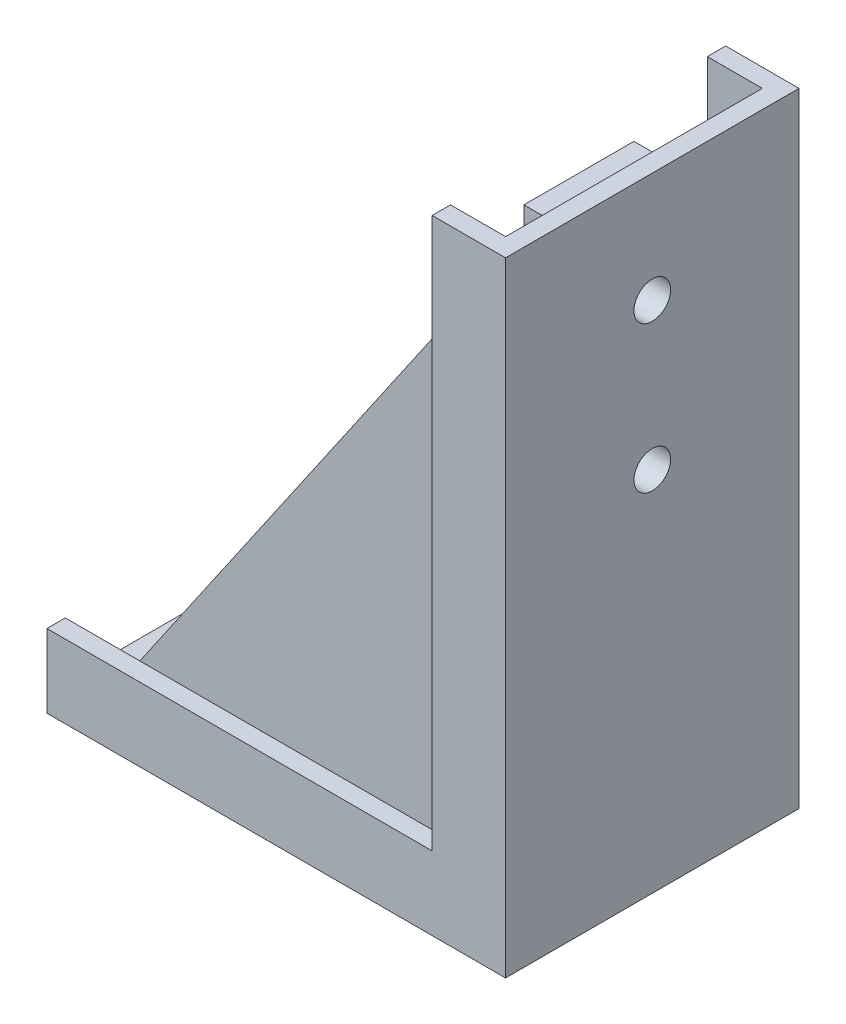
ISO-10303-21;
HEADER;
FILE_DESCRIPTION(('STEP AP214'),'2;1');
FILE_NAME('part.step','',(''),(''),'','','');
FILE_SCHEMA(('AUTOMOTIVE_DESIGN { 1 0 10303 214 1 1 1 1 }'));
ENDSEC;
DATA;
#1=APPLICATION_CONTEXT('core data for automotive mechanical design processes');
#2=APPLICATION_PROTOCOL_DEFINITION('international standard','automotive_design',2000,#1);
#3=PRODUCT_CONTEXT('',#1,'mechanical');
#4=PRODUCT('Part','Part','',(#3));
#5=PRODUCT_RELATED_PRODUCT_CATEGORY('part','',(#4));
#6=PRODUCT_DEFINITION_FORMATION('','',#4);
#7=PRODUCT_DEFINITION_CONTEXT('part definition',#1,'design');
#8=PRODUCT_DEFINITION('design','',#6,#7);
#9=PRODUCT_DEFINITION_SHAPE('','',#8);
#10=(LENGTH_UNIT() NAMED_UNIT(*) SI_UNIT(.MILLI.,.METRE.));
#11=(NAMED_UNIT(*) PLANE_ANGLE_UNIT() SI_UNIT($,.RADIAN.));
#12=(NAMED_UNIT(*) SI_UNIT($,.STERADIAN.) SOLID_ANGLE_UNIT());
#13=UNCERTAINTY_MEASURE_WITH_UNIT(LENGTH_MEASURE(1.E-05),#10,'distance_accuracy_value','');
#14=(GEOMETRIC_REPRESENTATION_CONTEXT(3) GLOBAL_UNCERTAINTY_ASSIGNED_CONTEXT((#13)) GLOBAL_UNIT_ASSIGNED_CONTEXT((#10,
#11,#12)) REPRESENTATION_CONTEXT('',''));
#15=CARTESIAN_POINT('',(0.,0.,0.));
#16=DIRECTION('',(0.,0.,1.));
#17=DIRECTION('',(1.,0.,0.));
#18=AXIS2_PLACEMENT_3D('',#15,#16,#17);
#19=CARTESIAN_POINT('',(-1.25,1.25,20.));
#20=DIRECTION('',(1.,0.,0.));
#21=DIRECTION('',(0.,1.,0.));
#22=AXIS2_PLACEMENT_3D('',#19,#20,#21);
#23=PLANE('',#22);
#24=DIRECTION('',(0.,-1.,0.));
#25=VECTOR('',#24,1.);
#26=CARTESIAN_POINT('',(-1.25,40.,6.25));
#27=LINE('',#26,#25);
#28=CARTESIAN_POINT('',(-1.25,40.,6.25));
#29=VERTEX_POINT('',#28);
#30=CARTESIAN_POINT('',(-1.25,17.5,6.25));
#31=VERTEX_POINT('',#30);
#32=EDGE_CURVE('E212',#29,#31,#27,.T.);
#33=ORIENTED_EDGE('',*,*,#32,.F.);
#34=DIRECTION('',(0.,0.,-1.));
#35=VECTOR('',#34,1.);
#36=CARTESIAN_POINT('',(-1.25,40.,6.25));
#37=LINE('',#36,#35);
#38=CARTESIAN_POINT('',(-1.25,40.,13.75));
#39=VERTEX_POINT('',#38);
#40=EDGE_CURVE('E206',#39,#29,#37,.T.);
#41=ORIENTED_EDGE('',*,*,#40,.F.);
#42=DIRECTION('',(0.,1.,0.));
#43=VECTOR('',#42,1.);
#44=CARTESIAN_POINT('',(-1.25,40.,13.75));
#45=LINE('',#44,#43);
#46=CARTESIAN_POINT('',(-1.25,17.5,13.75));
#47=VERTEX_POINT('',#46);
#48=EDGE_CURVE('E62',#47,#39,#45,.T.);
#49=ORIENTED_EDGE('',*,*,#48,.F.);
#50=DIRECTION('',(0.,0.,1.));
#51=VECTOR('',#50,1.);
#52=CARTESIAN_POINT('',(-1.25,17.5,6.25));
#53=LINE('',#52,#51);
#54=EDGE_CURVE('E57',#31,#47,#53,.T.);
#55=ORIENTED_EDGE('',*,*,#54,.F.);
#56=EDGE_LOOP('',(#33,#41,#49,#55));
#57=FACE_BOUND('',#56,.T.);
#58=DIRECTION('',(0.,0.,1.));
#59=VECTOR('',#58,1.);
#60=CARTESIAN_POINT('',(-1.25,41.25,17.5));
#61=LINE('',#60,#59);
#62=CARTESIAN_POINT('',(-1.25,41.25,17.5));
#63=VERTEX_POINT('',#62);
#64=CARTESIAN_POINT('',(-1.25,41.25,18.75));
#65=VERTEX_POINT('',#64);
#66=EDGE_CURVE('E228',#63,#65,#61,.T.);
#67=ORIENTED_EDGE('',*,*,#66,.T.);
#68=DIRECTION('',(0.,-1.,0.));
#69=VECTOR('',#68,1.);
#70=CARTESIAN_POINT('',(-1.25,42.5,18.75));
#71=LINE('',#70,#69);
#72=CARTESIAN_POINT('',(-1.25,42.5,18.75));
#73=VERTEX_POINT('',#72);
#74=EDGE_CURVE('E283',#73,#65,#71,.T.);
#75=ORIENTED_EDGE('',*,*,#74,.F.);
#76=DIRECTION('',(0.,0.,-1.));
#77=VECTOR('',#76,1.);
#78=CARTESIAN_POINT('',(-1.25,42.5,20.));
#79=LINE('',#78,#77);
#80=CARTESIAN_POINT('',(-1.25,42.5,1.25));
#81=VERTEX_POINT('',#80);
#82=EDGE_CURVE('E48',#73,#81,#79,.T.);
#83=ORIENTED_EDGE('',*,*,#82,.T.);
#84=DIRECTION('',(0.,-1.,0.));
#85=VECTOR('',#84,1.);
#86=CARTESIAN_POINT('',(-1.25,1.25,1.25));
#87=LINE('',#86,#85);
#88=CARTESIAN_POINT('',(-1.25,41.25,1.25));
#89=VERTEX_POINT('',#88);
#90=EDGE_CURVE('E278',#81,#89,#87,.T.);
#91=ORIENTED_EDGE('',*,*,#90,.T.);
#92=DIRECTION('',(0.,0.,-1.));
#93=VECTOR('',#92,1.);
#94=CARTESIAN_POINT('',(-1.25,41.25,2.5));
#95=LINE('',#94,#93);
#96=CARTESIAN_POINT('',(-1.25,41.25,2.5));
#97=VERTEX_POINT('',#96);
#98=EDGE_CURVE('E250',#97,#89,#95,.T.);
#99=ORIENTED_EDGE('',*,*,#98,.F.);
#100=DIRECTION('',(0.,-1.,0.));
#101=VECTOR('',#100,1.);
#102=CARTESIAN_POINT('',(-1.25,41.25,2.5));
#103=LINE('',#102,#101);
#104=CARTESIAN_POINT('',(-1.25,1.25,2.5));
#105=VERTEX_POINT('',#104);
#106=EDGE_CURVE('E239',#97,#105,#103,.T.);
#107=ORIENTED_EDGE('',*,*,#106,.T.);
#108=DIRECTION('',(0.,0.,-1.));
#109=VECTOR('',#108,1.);
#110=CARTESIAN_POINT('',(-1.25,1.25,20.));
#111=LINE('',#110,#109);
#112=CARTESIAN_POINT('',(-1.25,1.25,17.5));
#113=VERTEX_POINT('',#112);
#114=EDGE_CURVE('E341',#113,#105,#111,.T.);
#115=ORIENTED_EDGE('',*,*,#114,.F.);
#116=DIRECTION('',(0.,-1.,0.));
#117=VECTOR('',#116,1.);
#118=CARTESIAN_POINT('',(-1.25,1.25,17.5));
#119=LINE('',#118,#117);
#120=EDGE_CURVE('E221',#63,#113,#119,.T.);
#121=ORIENTED_EDGE('',*,*,#120,.F.);
#122=EDGE_LOOP('',(#67,#75,#83,#91,#99,#107,#115,#121));
#123=FACE_BOUND('',#122,.T.);
#124=ADVANCED_FACE('F39',(#57,#123),#23,.F.);
#125=CARTESIAN_POINT('',(-31.25,1.25,20.));
#126=DIRECTION('',(0.,-1.,0.));
#127=DIRECTION('',(1.,0.,0.));
#128=AXIS2_PLACEMENT_3D('',#125,#126,#127);
#129=PLANE('',#128);
#130=DIRECTION('',(0.,0.,1.));
#131=VECTOR('',#130,1.);
#132=CARTESIAN_POINT('',(-28.75,1.25,17.5));
#133=LINE('',#132,#131);
#134=CARTESIAN_POINT('',(-28.75,1.25,17.5));
#135=VERTEX_POINT('',#134);
#136=CARTESIAN_POINT('',(-28.75,1.25,18.75));
#137=VERTEX_POINT('',#136);
#138=EDGE_CURVE('E233',#135,#137,#133,.T.);
#139=ORIENTED_EDGE('',*,*,#138,.F.);
#140=DIRECTION('',(-1.,0.,0.));
#141=VECTOR('',#140,1.);
#142=CARTESIAN_POINT('',(-28.75,1.25,17.5));
#143=LINE('',#142,#141);
#144=EDGE_CURVE('E224',#113,#135,#143,.T.);
#145=ORIENTED_EDGE('',*,*,#144,.F.);
#146=ORIENTED_EDGE('',*,*,#114,.T.);
#147=DIRECTION('',(-1.,0.,0.));
#148=VECTOR('',#147,1.);
#149=CARTESIAN_POINT('',(-1.25,1.25,2.5));
#150=LINE('',#149,#148);
#151=CARTESIAN_POINT('',(-28.75,1.24999999999999,2.5));
#152=VERTEX_POINT('',#151);
#153=EDGE_CURVE('E234',#105,#152,#150,.T.);
#154=ORIENTED_EDGE('',*,*,#153,.T.);
#155=DIRECTION('',(0.,0.,-1.));
#156=VECTOR('',#155,1.);
#157=CARTESIAN_POINT('',(-28.75,1.24999999999999,2.5));
#158=LINE('',#157,#156);
#159=CARTESIAN_POINT('',(-28.75,1.24999999999999,1.25));
#160=VERTEX_POINT('',#159);
#161=EDGE_CURVE('E243',#152,#160,#158,.T.);
#162=ORIENTED_EDGE('',*,*,#161,.T.);
#163=DIRECTION('',(-1.,0.,0.));
#164=VECTOR('',#163,1.);
#165=CARTESIAN_POINT('',(-31.25,1.25,1.25));
#166=LINE('',#165,#164);
#167=CARTESIAN_POINT('',(-31.25,1.25,1.25));
#168=VERTEX_POINT('',#167);
#169=EDGE_CURVE('E274',#160,#168,#166,.T.);
#170=ORIENTED_EDGE('',*,*,#169,.T.);
#171=DIRECTION('',(0.,0.,-1.));
#172=VECTOR('',#171,1.);
#173=CARTESIAN_POINT('',(-31.25,1.25,20.));
#174=LINE('',#173,#172);
#175=CARTESIAN_POINT('',(-31.25,1.25,18.75));
#176=VERTEX_POINT('',#175);
#177=EDGE_CURVE('E342',#176,#168,#174,.T.);
#178=ORIENTED_EDGE('',*,*,#177,.F.);
#179=DIRECTION('',(-1.,0.,0.));
#180=VECTOR('',#179,1.);
#181=CARTESIAN_POINT('',(-1.25,1.25,18.75));
#182=LINE('',#181,#180);
#183=EDGE_CURVE('E287',#137,#176,#182,.T.);
#184=ORIENTED_EDGE('',*,*,#183,.F.);
#185=EDGE_LOOP('',(#139,#145,#146,#154,#162,#170,#178,#184));
#186=FACE_BOUND('',#185,.T.);
#187=ADVANCED_FACE('F387',(#186),#129,.F.);
#188=CARTESIAN_POINT('',(0.,0.,18.75));
#189=DIRECTION('',(0.,0.,-1.));
#190=DIRECTION('',(-1.,0.,0.));
#191=AXIS2_PLACEMENT_3D('',#188,#189,#190);
#192=PLANE('',#191);
#193=ORIENTED_EDGE('',*,*,#74,.T.);
#194=DIRECTION('',(-0.566528822887065,-0.824041924199368,0.));
#195=VECTOR('',#194,1.);
#196=CARTESIAN_POINT('',(-20.106100795756,13.8229442970822,18.75));
#197=LINE('',#196,#195);
#198=CARTESIAN_POINT('',(-5.,35.7954545454545,18.75));
#199=VERTEX_POINT('',#198);
#200=EDGE_CURVE('E11',#65,#199,#197,.T.);
#201=ORIENTED_EDGE('',*,*,#200,.T.);
#202=DIRECTION('',(0.,-1.,0.));
#203=VECTOR('',#202,1.);
#204=CARTESIAN_POINT('',(-5.,42.5,18.75));
#205=LINE('',#204,#203);
#206=CARTESIAN_POINT('',(-5.,42.5,18.75));
#207=VERTEX_POINT('',#206);
#208=EDGE_CURVE('E296',#207,#199,#205,.T.);
#209=ORIENTED_EDGE('',*,*,#208,.F.);
#210=DIRECTION('',(-1.,0.,0.));
#211=VECTOR('',#210,1.);
#212=CARTESIAN_POINT('',(-1.25,42.5,18.75));
#213=LINE('',#212,#211);
#214=EDGE_CURVE('E301',#73,#207,#213,.T.);
#215=ORIENTED_EDGE('',*,*,#214,.F.);
#216=EDGE_LOOP('',(#193,#201,#209,#215));
#217=FACE_BOUND('',#216,.T.);
#218=ADVANCED_FACE('F395',(#217),#192,.T.);
#219=DIRECTION('',(-1.,0.,0.));
#220=VECTOR('',#219,1.);
#221=CARTESIAN_POINT('',(-5.,5.,18.75));
#222=LINE('',#221,#220);
#223=CARTESIAN_POINT('',(-26.171875,5.,18.75));
#224=VERTEX_POINT('',#223);
#225=CARTESIAN_POINT('',(-31.25,5.,18.75));
#226=VERTEX_POINT('',#225);
#227=EDGE_CURVE('E291',#224,#226,#222,.T.);
#228=ORIENTED_EDGE('',*,*,#227,.F.);
#229=DIRECTION('',(0.566528822887065,0.824041924199368,0.));
#230=VECTOR('',#229,1.);
#231=CARTESIAN_POINT('',(-1.25,41.25,18.75));
#232=LINE('',#231,#230);
#233=EDGE_CURVE('E213',#137,#224,#232,.T.);
#234=ORIENTED_EDGE('',*,*,#233,.F.);
#235=ORIENTED_EDGE('',*,*,#183,.T.);
#236=DIRECTION('',(0.,-1.,0.));
#237=VECTOR('',#236,1.);
#238=CARTESIAN_POINT('',(-31.25,5.,18.75));
#239=LINE('',#238,#237);
#240=EDGE_CURVE('E290',#226,#176,#239,.T.);
#241=ORIENTED_EDGE('',*,*,#240,.F.);
#242=EDGE_LOOP('',(#228,#234,#235,#241));
#243=FACE_BOUND('',#242,.T.);
#244=ADVANCED_FACE('F430',(#243),#192,.T.);
#245=CARTESIAN_POINT('',(0.,0.,1.25));
#246=DIRECTION('',(0.,0.,1.));
#247=DIRECTION('',(1.,0.,0.));
#248=AXIS2_PLACEMENT_3D('',#245,#246,#247);
#249=PLANE('',#248);
#250=DIRECTION('',(0.566528822887065,0.824041924199368,0.));
#251=VECTOR('',#250,1.);
#252=CARTESIAN_POINT('',(-28.75,1.24999999999999,1.25));
#253=LINE('',#252,#251);
#254=CARTESIAN_POINT('',(-5.,35.7954545454545,1.25));
#255=VERTEX_POINT('',#254);
#256=EDGE_CURVE('E231',#255,#89,#253,.T.);
#257=ORIENTED_EDGE('',*,*,#256,.T.);
#258=ORIENTED_EDGE('',*,*,#90,.F.);
#259=DIRECTION('',(1.,0.,0.));
#260=VECTOR('',#259,1.);
#261=CARTESIAN_POINT('',(-1.25,42.5,1.25));
#262=LINE('',#261,#260);
#263=CARTESIAN_POINT('',(-5.,42.5,1.25));
#264=VERTEX_POINT('',#263);
#265=EDGE_CURVE('E262',#264,#81,#262,.T.);
#266=ORIENTED_EDGE('',*,*,#265,.F.);
#267=DIRECTION('',(0.,1.,0.));
#268=VECTOR('',#267,1.);
#269=CARTESIAN_POINT('',(-5.,42.5,1.25));
#270=LINE('',#269,#268);
#271=EDGE_CURVE('E256',#255,#264,#270,.T.);
#272=ORIENTED_EDGE('',*,*,#271,.F.);
#273=EDGE_LOOP('',(#257,#258,#266,#272));
#274=FACE_BOUND('',#273,.T.);
#275=ADVANCED_FACE('F441',(#274),#249,.T.);
#276=CARTESIAN_POINT('',(-1.25,42.5,20.));
#277=DIRECTION('',(0.,-1.,0.));
#278=DIRECTION('',(0.,0.,-1.));
#279=AXIS2_PLACEMENT_3D('',#276,#277,#278);
#280=PLANE('',#279);
#281=DIRECTION('',(0.,0.,-1.));
#282=VECTOR('',#281,1.);
#283=CARTESIAN_POINT('',(0.,42.5,20.));
#284=LINE('',#283,#282);
#285=CARTESIAN_POINT('',(0.,42.5,20.));
#286=VERTEX_POINT('',#285);
#287=CARTESIAN_POINT('',(0.,42.5,0.));
#288=VERTEX_POINT('',#287);
#289=EDGE_CURVE('E326',#286,#288,#284,.T.);
#290=ORIENTED_EDGE('',*,*,#289,.T.);
#291=DIRECTION('',(-1.,0.,0.));
#292=VECTOR('',#291,1.);
#293=CARTESIAN_POINT('',(-1.25,42.5,0.));
#294=LINE('',#293,#292);
#295=CARTESIAN_POINT('',(-5.,42.5,0.));
#296=VERTEX_POINT('',#295);
#297=EDGE_CURVE('E317',#288,#296,#294,.T.);
#298=ORIENTED_EDGE('',*,*,#297,.T.);
#299=DIRECTION('',(0.,0.,-1.));
#300=VECTOR('',#299,1.);
#301=CARTESIAN_POINT('',(-5.,42.5,1.25));
#302=LINE('',#301,#300);
#303=EDGE_CURVE('E272',#264,#296,#302,.T.);
#304=ORIENTED_EDGE('',*,*,#303,.F.);
#305=ORIENTED_EDGE('',*,*,#265,.T.);
#306=ORIENTED_EDGE('',*,*,#82,.F.);
#307=ORIENTED_EDGE('',*,*,#214,.T.);
#308=DIRECTION('',(0.,0.,1.));
#309=VECTOR('',#308,1.);
#310=CARTESIAN_POINT('',(-5.,42.5,18.75));
#311=LINE('',#310,#309);
#312=CARTESIAN_POINT('',(-5.,42.5,20.));
#313=VERTEX_POINT('',#312);
#314=EDGE_CURVE('E302',#207,#313,#311,.T.);
#315=ORIENTED_EDGE('',*,*,#314,.T.);
#316=DIRECTION('',(-1.,0.,0.));
#317=VECTOR('',#316,1.);
#318=CARTESIAN_POINT('',(-1.25,42.5,20.));
#319=LINE('',#318,#317);
#320=EDGE_CURVE('E320',#286,#313,#319,.T.);
#321=ORIENTED_EDGE('',*,*,#320,.F.);
#322=EDGE_LOOP('',(#290,#298,#304,#305,#306,#307,#315,#321));
#323=FACE_BOUND('',#322,.T.);
#324=ADVANCED_FACE('F41',(#323),#280,.F.);
#325=CARTESIAN_POINT('',(-31.25,0.,20.));
#326=DIRECTION('',(1.,0.,0.));
#327=DIRECTION('',(0.,0.,-1.));
#328=AXIS2_PLACEMENT_3D('',#325,#326,#327);
#329=PLANE('',#328);
#330=ORIENTED_EDGE('',*,*,#177,.T.);
#331=DIRECTION('',(0.,1.,0.));
#332=VECTOR('',#331,1.);
#333=CARTESIAN_POINT('',(-31.25,1.25,1.25));
#334=LINE('',#333,#332);
#335=CARTESIAN_POINT('',(-31.25,5.,1.25));
#336=VERTEX_POINT('',#335);
#337=EDGE_CURVE('E255',#168,#336,#334,.T.);
#338=ORIENTED_EDGE('',*,*,#337,.T.);
#339=DIRECTION('',(0.,0.,-1.));
#340=VECTOR('',#339,1.);
#341=CARTESIAN_POINT('',(-31.25,5.,1.25));
#342=LINE('',#341,#340);
#343=CARTESIAN_POINT('',(-31.25,5.,0.));
#344=VERTEX_POINT('',#343);
#345=EDGE_CURVE('E266',#336,#344,#342,.T.);
#346=ORIENTED_EDGE('',*,*,#345,.T.);
#347=DIRECTION('',(0.,-1.,0.));
#348=VECTOR('',#347,1.);
#349=CARTESIAN_POINT('',(-31.25,0.,0.));
#350=LINE('',#349,#348);
#351=CARTESIAN_POINT('',(-31.25,0.,0.));
#352=VERTEX_POINT('',#351);
#353=EDGE_CURVE('E327',#344,#352,#350,.T.);
#354=ORIENTED_EDGE('',*,*,#353,.T.);
#355=DIRECTION('',(0.,0.,-1.));
#356=VECTOR('',#355,1.);
#357=CARTESIAN_POINT('',(-31.25,0.,20.));
#358=LINE('',#357,#356);
#359=CARTESIAN_POINT('',(-31.25,0.,20.));
#360=VERTEX_POINT('',#359);
#361=EDGE_CURVE('E339',#360,#352,#358,.T.);
#362=ORIENTED_EDGE('',*,*,#361,.F.);
#363=DIRECTION('',(0.,-1.,0.));
#364=VECTOR('',#363,1.);
#365=CARTESIAN_POINT('',(-31.25,0.,20.));
#366=LINE('',#365,#364);
#367=CARTESIAN_POINT('',(-31.25,5.,20.));
#368=VERTEX_POINT('',#367);
#369=EDGE_CURVE('E316',#368,#360,#366,.T.);
#370=ORIENTED_EDGE('',*,*,#369,.F.);
#371=DIRECTION('',(0.,0.,1.));
#372=VECTOR('',#371,1.);
#373=CARTESIAN_POINT('',(-31.25,5.,18.75));
#374=LINE('',#373,#372);
#375=EDGE_CURVE('E312',#226,#368,#374,.T.);
#376=ORIENTED_EDGE('',*,*,#375,.F.);
#377=ORIENTED_EDGE('',*,*,#240,.T.);
#378=EDGE_LOOP('',(#330,#338,#346,#354,#362,#370,#376,#377));
#379=FACE_BOUND('',#378,.T.);
#380=ADVANCED_FACE('F397',(#379),#329,.F.);
#381=CARTESIAN_POINT('',(0.,0.,20.));
#382=DIRECTION('',(0.,1.,0.));
#383=DIRECTION('',(0.,0.,1.));
#384=AXIS2_PLACEMENT_3D('',#381,#382,#383);
#385=PLANE('',#384);
#386=ORIENTED_EDGE('',*,*,#361,.T.);
#387=DIRECTION('',(1.,0.,0.));
#388=VECTOR('',#387,1.);
#389=CARTESIAN_POINT('',(0.,0.,0.));
#390=LINE('',#389,#388);
#391=CARTESIAN_POINT('',(0.,0.,0.));
#392=VERTEX_POINT('',#391);
#393=EDGE_CURVE('E331',#352,#392,#390,.T.);
#394=ORIENTED_EDGE('',*,*,#393,.T.);
#395=DIRECTION('',(0.,0.,-1.));
#396=VECTOR('',#395,1.);
#397=CARTESIAN_POINT('',(0.,0.,20.));
#398=LINE('',#397,#396);
#399=CARTESIAN_POINT('',(0.,0.,20.));
#400=VERTEX_POINT('',#399);
#401=EDGE_CURVE('E340',#400,#392,#398,.T.);
#402=ORIENTED_EDGE('',*,*,#401,.F.);
#403=DIRECTION('',(1.,0.,0.));
#404=VECTOR('',#403,1.);
#405=CARTESIAN_POINT('',(0.,0.,20.));
#406=LINE('',#405,#404);
#407=EDGE_CURVE('E325',#360,#400,#406,.T.);
#408=ORIENTED_EDGE('',*,*,#407,.F.);
#409=EDGE_LOOP('',(#386,#394,#402,#408));
#410=FACE_BOUND('',#409,.T.);
#411=ADVANCED_FACE('F400',(#410),#385,.F.);
#412=CARTESIAN_POINT('',(0.,42.5,20.));
#413=DIRECTION('',(-1.,0.,0.));
#414=DIRECTION('',(0.,-1.,0.));
#415=AXIS2_PLACEMENT_3D('',#412,#413,#414);
#416=PLANE('',#415);
#417=CARTESIAN_POINT('',(0.,35.,10.));
#418=DIRECTION('',(-1.,0.,0.));
#419=DIRECTION('',(0.,-1.,0.));
#420=AXIS2_PLACEMENT_3D('',#417,#418,#419);
#421=CIRCLE('',#420,1.25);
#422=CARTESIAN_POINT('',(0.,33.75,10.));
#423=VERTEX_POINT('',#422);
#424=EDGE_CURVE('E43',#423,#423,#421,.T.);
#425=ORIENTED_EDGE('',*,*,#424,.T.);
#426=EDGE_LOOP('',(#425));
#427=FACE_BOUND('',#426,.T.);
#428=CARTESIAN_POINT('',(0.,25.,10.));
#429=DIRECTION('',(-1.,0.,0.));
#430=DIRECTION('',(0.,-1.,0.));
#431=AXIS2_PLACEMENT_3D('',#428,#429,#430);
#432=CIRCLE('',#431,1.25);
#433=CARTESIAN_POINT('',(0.,23.75,10.));
#434=VERTEX_POINT('',#433);
#435=EDGE_CURVE('E346',#434,#434,#432,.T.);
#436=ORIENTED_EDGE('',*,*,#435,.T.);
#437=EDGE_LOOP('',(#436));
#438=FACE_BOUND('',#437,.T.);
#439=ORIENTED_EDGE('',*,*,#401,.T.);
#440=DIRECTION('',(0.,1.,0.));
#441=VECTOR('',#440,1.);
#442=CARTESIAN_POINT('',(0.,42.5,0.));
#443=LINE('',#442,#441);
#444=EDGE_CURVE('E318',#392,#288,#443,.T.);
#445=ORIENTED_EDGE('',*,*,#444,.T.);
#446=ORIENTED_EDGE('',*,*,#289,.F.);
#447=DIRECTION('',(0.,1.,0.));
#448=VECTOR('',#447,1.);
#449=CARTESIAN_POINT('',(0.,42.5,20.));
#450=LINE('',#449,#448);
#451=EDGE_CURVE('E321',#400,#286,#450,.T.);
#452=ORIENTED_EDGE('',*,*,#451,.F.);
#453=EDGE_LOOP('',(#439,#445,#446,#452));
#454=FACE_BOUND('',#453,.T.);
#455=ADVANCED_FACE('F404',(#427,#438,#454),#416,.F.);
#456=CARTESIAN_POINT('',(0.,0.,20.));
#457=DIRECTION('',(0.,0.,-1.));
#458=DIRECTION('',(-1.,0.,0.));
#459=AXIS2_PLACEMENT_3D('',#456,#457,#458);
#460=PLANE('',#459);
#461=ORIENTED_EDGE('',*,*,#320,.T.);
#462=DIRECTION('',(0.,-1.,0.));
#463=VECTOR('',#462,1.);
#464=CARTESIAN_POINT('',(-5.,42.5,20.));
#465=LINE('',#464,#463);
#466=CARTESIAN_POINT('',(-5.,5.,20.));
#467=VERTEX_POINT('',#466);
#468=EDGE_CURVE('E289',#313,#467,#465,.T.);
#469=ORIENTED_EDGE('',*,*,#468,.T.);
#470=DIRECTION('',(-1.,0.,0.));
#471=VECTOR('',#470,1.);
#472=CARTESIAN_POINT('',(-5.,5.,20.));
#473=LINE('',#472,#471);
#474=EDGE_CURVE('E282',#467,#368,#473,.T.);
#475=ORIENTED_EDGE('',*,*,#474,.T.);
#476=ORIENTED_EDGE('',*,*,#369,.T.);
#477=ORIENTED_EDGE('',*,*,#407,.T.);
#478=ORIENTED_EDGE('',*,*,#451,.T.);
#479=EDGE_LOOP('',(#461,#469,#475,#476,#477,#478));
#480=FACE_BOUND('',#479,.T.);
#481=ADVANCED_FACE('F409',(#480),#460,.F.);
#482=CARTESIAN_POINT('',(0.,0.,0.));
#483=DIRECTION('',(0.,0.,-1.));
#484=DIRECTION('',(-1.,0.,0.));
#485=AXIS2_PLACEMENT_3D('',#482,#483,#484);
#486=PLANE('',#485);
#487=ORIENTED_EDGE('',*,*,#297,.F.);
#488=ORIENTED_EDGE('',*,*,#444,.F.);
#489=ORIENTED_EDGE('',*,*,#393,.F.);
#490=ORIENTED_EDGE('',*,*,#353,.F.);
#491=DIRECTION('',(1.,0.,0.));
#492=VECTOR('',#491,1.);
#493=CARTESIAN_POINT('',(-5.,5.,0.));
#494=LINE('',#493,#492);
#495=CARTESIAN_POINT('',(-5.,5.,0.));
#496=VERTEX_POINT('',#495);
#497=EDGE_CURVE('E248',#344,#496,#494,.T.);
#498=ORIENTED_EDGE('',*,*,#497,.T.);
#499=DIRECTION('',(0.,1.,0.));
#500=VECTOR('',#499,1.);
#501=CARTESIAN_POINT('',(-5.,42.5,0.));
#502=LINE('',#501,#500);
#503=EDGE_CURVE('E253',#496,#296,#502,.T.);
#504=ORIENTED_EDGE('',*,*,#503,.T.);
#505=EDGE_LOOP('',(#487,#488,#489,#490,#498,#504));
#506=FACE_BOUND('',#505,.T.);
#507=ADVANCED_FACE('F406',(#506),#486,.T.);
#508=CARTESIAN_POINT('',(-5.,5.,18.75));
#509=DIRECTION('',(0.,1.,0.));
#510=DIRECTION('',(-1.,0.,0.));
#511=AXIS2_PLACEMENT_3D('',#508,#509,#510);
#512=PLANE('',#511);
#513=ORIENTED_EDGE('',*,*,#474,.F.);
#514=DIRECTION('',(0.,0.,1.));
#515=VECTOR('',#514,1.);
#516=CARTESIAN_POINT('',(-5.,5.,18.75));
#517=LINE('',#516,#515);
#518=CARTESIAN_POINT('',(-5.,5.,18.75));
#519=VERTEX_POINT('',#518);
#520=EDGE_CURVE('E311',#519,#467,#517,.T.);
#521=ORIENTED_EDGE('',*,*,#520,.F.);
#522=EDGE_CURVE('E295',#519,#224,#222,.T.);
#523=ORIENTED_EDGE('',*,*,#522,.T.);
#524=ORIENTED_EDGE('',*,*,#227,.T.);
#525=ORIENTED_EDGE('',*,*,#375,.T.);
#526=EDGE_LOOP('',(#513,#521,#523,#524,#525));
#527=FACE_BOUND('',#526,.T.);
#528=ADVANCED_FACE('F415',(#527),#512,.T.);
#529=CARTESIAN_POINT('',(-5.,42.5,18.75));
#530=DIRECTION('',(-1.,0.,0.));
#531=DIRECTION('',(0.,-1.,0.));
#532=AXIS2_PLACEMENT_3D('',#529,#530,#531);
#533=PLANE('',#532);
#534=ORIENTED_EDGE('',*,*,#468,.F.);
#535=ORIENTED_EDGE('',*,*,#314,.F.);
#536=ORIENTED_EDGE('',*,*,#208,.T.);
#537=EDGE_CURVE('E300',#199,#519,#205,.T.);
#538=ORIENTED_EDGE('',*,*,#537,.T.);
#539=ORIENTED_EDGE('',*,*,#520,.T.);
#540=EDGE_LOOP('',(#534,#535,#536,#538,#539));
#541=FACE_BOUND('',#540,.T.);
#542=ADVANCED_FACE('F418',(#541),#533,.T.);
#543=CARTESIAN_POINT('',(-26.171875,5.,1.25));
#544=VERTEX_POINT('',#543);
#545=EDGE_CURVE('E238',#160,#544,#253,.T.);
#546=ORIENTED_EDGE('',*,*,#545,.T.);
#547=DIRECTION('',(1.,0.,0.));
#548=VECTOR('',#547,1.);
#549=CARTESIAN_POINT('',(-5.,5.,1.25));
#550=LINE('',#549,#548);
#551=EDGE_CURVE('E257',#336,#544,#550,.T.);
#552=ORIENTED_EDGE('',*,*,#551,.F.);
#553=ORIENTED_EDGE('',*,*,#337,.F.);
#554=ORIENTED_EDGE('',*,*,#169,.F.);
#555=EDGE_LOOP('',(#546,#552,#553,#554));
#556=FACE_BOUND('',#555,.T.);
#557=ADVANCED_FACE('F421',(#556),#249,.T.);
#558=CARTESIAN_POINT('',(-5.,42.5,1.25));
#559=DIRECTION('',(-1.,0.,0.));
#560=DIRECTION('',(0.,-1.,0.));
#561=AXIS2_PLACEMENT_3D('',#558,#559,#560);
#562=PLANE('',#561);
#563=ORIENTED_EDGE('',*,*,#503,.F.);
#564=DIRECTION('',(0.,0.,-1.));
#565=VECTOR('',#564,1.);
#566=CARTESIAN_POINT('',(-5.,5.,1.25));
#567=LINE('',#566,#565);
#568=CARTESIAN_POINT('',(-5.,5.,1.25));
#569=VERTEX_POINT('',#568);
#570=EDGE_CURVE('E273',#569,#496,#567,.T.);
#571=ORIENTED_EDGE('',*,*,#570,.F.);
#572=EDGE_CURVE('E258',#569,#255,#270,.T.);
#573=ORIENTED_EDGE('',*,*,#572,.T.);
#574=ORIENTED_EDGE('',*,*,#271,.T.);
#575=ORIENTED_EDGE('',*,*,#303,.T.);
#576=EDGE_LOOP('',(#563,#571,#573,#574,#575));
#577=FACE_BOUND('',#576,.T.);
#578=ADVANCED_FACE('F433',(#577),#562,.T.);
#579=CARTESIAN_POINT('',(-5.,5.,1.25));
#580=DIRECTION('',(0.,1.,0.));
#581=DIRECTION('',(-1.,0.,0.));
#582=AXIS2_PLACEMENT_3D('',#579,#580,#581);
#583=PLANE('',#582);
#584=ORIENTED_EDGE('',*,*,#497,.F.);
#585=ORIENTED_EDGE('',*,*,#345,.F.);
#586=ORIENTED_EDGE('',*,*,#551,.T.);
#587=EDGE_CURVE('E251',#544,#569,#550,.T.);
#588=ORIENTED_EDGE('',*,*,#587,.T.);
#589=ORIENTED_EDGE('',*,*,#570,.T.);
#590=EDGE_LOOP('',(#584,#585,#586,#588,#589));
#591=FACE_BOUND('',#590,.T.);
#592=ADVANCED_FACE('F429',(#591),#583,.T.);
#593=CARTESIAN_POINT('',(-28.75,1.24999999999999,2.5));
#594=DIRECTION('',(-0.824041924199368,0.566528822887065,0.));
#595=DIRECTION('',(-0.566528822887065,-0.824041924199368,0.));
#596=AXIS2_PLACEMENT_3D('',#593,#594,#595);
#597=PLANE('',#596);
#598=ORIENTED_EDGE('',*,*,#545,.F.);
#599=ORIENTED_EDGE('',*,*,#161,.F.);
#600=DIRECTION('',(0.566528822887065,0.824041924199368,0.));
#601=VECTOR('',#600,1.);
#602=CARTESIAN_POINT('',(-28.75,1.24999999999999,2.5));
#603=LINE('',#602,#601);
#604=EDGE_CURVE('E240',#152,#97,#603,.T.);
#605=ORIENTED_EDGE('',*,*,#604,.T.);
#606=ORIENTED_EDGE('',*,*,#98,.T.);
#607=ORIENTED_EDGE('',*,*,#256,.F.);
#608=EDGE_CURVE('E246',#544,#255,#253,.T.);
#609=ORIENTED_EDGE('',*,*,#608,.F.);
#610=EDGE_LOOP('',(#598,#599,#605,#606,#607,#609));
#611=FACE_BOUND('',#610,.T.);
#612=ADVANCED_FACE('F435',(#611),#597,.T.);
#613=CARTESIAN_POINT('',(0.,0.,2.5));
#614=DIRECTION('',(0.,0.,1.));
#615=DIRECTION('',(1.,0.,0.));
#616=AXIS2_PLACEMENT_3D('',#613,#614,#615);
#617=PLANE('',#616);
#618=ORIENTED_EDGE('',*,*,#153,.F.);
#619=ORIENTED_EDGE('',*,*,#106,.F.);
#620=ORIENTED_EDGE('',*,*,#604,.F.);
#621=EDGE_LOOP('',(#618,#619,#620));
#622=FACE_BOUND('',#621,.T.);
#623=ADVANCED_FACE('F443',(#622),#617,.T.);
#624=CARTESIAN_POINT('',(0.,0.,1.25));
#625=DIRECTION('',(0.,0.,1.));
#626=DIRECTION('',(1.,0.,0.));
#627=AXIS2_PLACEMENT_3D('',#624,#625,#626);
#628=PLANE('',#627);
#629=ORIENTED_EDGE('',*,*,#572,.F.);
#630=ORIENTED_EDGE('',*,*,#587,.F.);
#631=ORIENTED_EDGE('',*,*,#608,.T.);
#632=EDGE_LOOP('',(#629,#630,#631));
#633=FACE_BOUND('',#632,.T.);
#634=ADVANCED_FACE('F447',(#633),#628,.F.);
#635=CARTESIAN_POINT('',(-1.25,41.25,17.5));
#636=DIRECTION('',(0.824041924199368,-0.566528822887065,0.));
#637=DIRECTION('',(0.566528822887065,0.824041924199368,0.));
#638=AXIS2_PLACEMENT_3D('',#635,#636,#637);
#639=PLANE('',#638);
#640=ORIENTED_EDGE('',*,*,#233,.T.);
#641=EDGE_CURVE('E215',#224,#199,#232,.T.);
#642=ORIENTED_EDGE('',*,*,#641,.T.);
#643=ORIENTED_EDGE('',*,*,#200,.F.);
#644=ORIENTED_EDGE('',*,*,#66,.F.);
#645=DIRECTION('',(0.566528822887065,0.824041924199368,0.));
#646=VECTOR('',#645,1.);
#647=CARTESIAN_POINT('',(-1.25,41.25,17.5));
#648=LINE('',#647,#646);
#649=EDGE_CURVE('E225',#135,#63,#648,.T.);
#650=ORIENTED_EDGE('',*,*,#649,.F.);
#651=ORIENTED_EDGE('',*,*,#138,.T.);
#652=EDGE_LOOP('',(#640,#642,#643,#644,#650,#651));
#653=FACE_BOUND('',#652,.T.);
#654=ADVANCED_FACE('F446',(#653),#639,.F.);
#655=CARTESIAN_POINT('',(0.,0.,17.5));
#656=DIRECTION('',(0.,0.,-1.));
#657=DIRECTION('',(-1.,0.,0.));
#658=AXIS2_PLACEMENT_3D('',#655,#656,#657);
#659=PLANE('',#658);
#660=ORIENTED_EDGE('',*,*,#120,.T.);
#661=ORIENTED_EDGE('',*,*,#144,.T.);
#662=ORIENTED_EDGE('',*,*,#649,.T.);
#663=EDGE_LOOP('',(#660,#661,#662));
#664=FACE_BOUND('',#663,.T.);
#665=ADVANCED_FACE('F456',(#664),#659,.T.);
#666=CARTESIAN_POINT('',(0.,0.,18.75));
#667=DIRECTION('',(0.,0.,-1.));
#668=DIRECTION('',(-1.,0.,0.));
#669=AXIS2_PLACEMENT_3D('',#666,#667,#668);
#670=PLANE('',#669);
#671=ORIENTED_EDGE('',*,*,#522,.F.);
#672=ORIENTED_EDGE('',*,*,#537,.F.);
#673=ORIENTED_EDGE('',*,*,#641,.F.);
#674=EDGE_LOOP('',(#671,#672,#673));
#675=FACE_BOUND('',#674,.T.);
#676=ADVANCED_FACE('F457',(#675),#670,.F.);
#677=CARTESIAN_POINT('',(-5.,0.,0.));
#678=DIRECTION('',(-1.,0.,0.));
#679=DIRECTION('',(0.,-1.,0.));
#680=AXIS2_PLACEMENT_3D('',#677,#678,#679);
#681=PLANE('',#680);
#682=CARTESIAN_POINT('',(-5.,35.,10.));
#683=DIRECTION('',(-1.,0.,0.));
#684=DIRECTION('',(0.,-1.,0.));
#685=AXIS2_PLACEMENT_3D('',#682,#683,#684);
#686=CIRCLE('',#685,1.25);
#687=CARTESIAN_POINT('',(-5.,33.75,10.));
#688=VERTEX_POINT('',#687);
#689=EDGE_CURVE('E355',#688,#688,#686,.T.);
#690=ORIENTED_EDGE('',*,*,#689,.F.);
#691=EDGE_LOOP('',(#690));
#692=FACE_BOUND('',#691,.T.);
#693=DIRECTION('',(0.,-1.,0.));
#694=VECTOR('',#693,1.);
#695=CARTESIAN_POINT('',(-5.,40.,6.25));
#696=LINE('',#695,#694);
#697=CARTESIAN_POINT('',(-5.,40.,6.25));
#698=VERTEX_POINT('',#697);
#699=CARTESIAN_POINT('',(-5.,17.5,6.25));
#700=VERTEX_POINT('',#699);
#701=EDGE_CURVE('E197',#698,#700,#696,.T.);
#702=ORIENTED_EDGE('',*,*,#701,.T.);
#703=DIRECTION('',(0.,0.,1.));
#704=VECTOR('',#703,1.);
#705=CARTESIAN_POINT('',(-5.,17.5,6.25));
#706=LINE('',#705,#704);
#707=CARTESIAN_POINT('',(-5.,17.5,13.75));
#708=VERTEX_POINT('',#707);
#709=EDGE_CURVE('E190',#700,#708,#706,.T.);
#710=ORIENTED_EDGE('',*,*,#709,.T.);
#711=DIRECTION('',(0.,1.,0.));
#712=VECTOR('',#711,1.);
#713=CARTESIAN_POINT('',(-5.,40.,13.75));
#714=LINE('',#713,#712);
#715=CARTESIAN_POINT('',(-5.,40.,13.75));
#716=VERTEX_POINT('',#715);
#717=EDGE_CURVE('E200',#708,#716,#714,.T.);
#718=ORIENTED_EDGE('',*,*,#717,.T.);
#719=DIRECTION('',(0.,0.,-1.));
#720=VECTOR('',#719,1.);
#721=CARTESIAN_POINT('',(-5.,40.,6.25));
#722=LINE('',#721,#720);
#723=EDGE_CURVE('E203',#716,#698,#722,.T.);
#724=ORIENTED_EDGE('',*,*,#723,.T.);
#725=EDGE_LOOP('',(#702,#710,#718,#724));
#726=FACE_BOUND('',#725,.T.);
#727=CARTESIAN_POINT('',(-5.,25.,10.));
#728=DIRECTION('',(-1.,0.,0.));
#729=DIRECTION('',(0.,-1.,0.));
#730=AXIS2_PLACEMENT_3D('',#727,#728,#729);
#731=CIRCLE('',#730,1.25);
#732=CARTESIAN_POINT('',(-5.,23.75,10.));
#733=VERTEX_POINT('',#732);
#734=EDGE_CURVE('E351',#733,#733,#731,.T.);
#735=ORIENTED_EDGE('',*,*,#734,.F.);
#736=EDGE_LOOP('',(#735));
#737=FACE_BOUND('',#736,.T.);
#738=ADVANCED_FACE('F201',(#692,#726,#737),#681,.T.);
#739=CARTESIAN_POINT('',(-5.,40.,6.25));
#740=DIRECTION('',(0.,0.,1.));
#741=DIRECTION('',(0.,-1.,0.));
#742=AXIS2_PLACEMENT_3D('',#739,#740,#741);
#743=PLANE('',#742);
#744=ORIENTED_EDGE('',*,*,#32,.T.);
#745=DIRECTION('',(1.,0.,0.));
#746=VECTOR('',#745,1.);
#747=CARTESIAN_POINT('',(-5.,17.5,6.25));
#748=LINE('',#747,#746);
#749=EDGE_CURVE('E192',#700,#31,#748,.T.);
#750=ORIENTED_EDGE('',*,*,#749,.F.);
#751=ORIENTED_EDGE('',*,*,#701,.F.);
#752=DIRECTION('',(1.,0.,0.));
#753=VECTOR('',#752,1.);
#754=CARTESIAN_POINT('',(-5.,40.,6.25));
#755=LINE('',#754,#753);
#756=EDGE_CURVE('E364',#698,#29,#755,.T.);
#757=ORIENTED_EDGE('',*,*,#756,.T.);
#758=EDGE_LOOP('',(#744,#750,#751,#757));
#759=FACE_BOUND('',#758,.T.);
#760=ADVANCED_FACE('F208',(#759),#743,.F.);
#761=CARTESIAN_POINT('',(-5.,17.5,6.25));
#762=DIRECTION('',(0.,1.,0.));
#763=DIRECTION('',(-1.,0.,0.));
#764=AXIS2_PLACEMENT_3D('',#761,#762,#763);
#765=PLANE('',#764);
#766=ORIENTED_EDGE('',*,*,#54,.T.);
#767=DIRECTION('',(1.,0.,0.));
#768=VECTOR('',#767,1.);
#769=CARTESIAN_POINT('',(-5.,17.5,13.75));
#770=LINE('',#769,#768);
#771=EDGE_CURVE('E191',#708,#47,#770,.T.);
#772=ORIENTED_EDGE('',*,*,#771,.F.);
#773=ORIENTED_EDGE('',*,*,#709,.F.);
#774=ORIENTED_EDGE('',*,*,#749,.T.);
#775=EDGE_LOOP('',(#766,#772,#773,#774));
#776=FACE_BOUND('',#775,.T.);
#777=ADVANCED_FACE('F186',(#776),#765,.F.);
#778=CARTESIAN_POINT('',(-5.,40.,13.75));
#779=DIRECTION('',(0.,0.,-1.));
#780=DIRECTION('',(0.,1.,0.));
#781=AXIS2_PLACEMENT_3D('',#778,#779,#780);
#782=PLANE('',#781);
#783=ORIENTED_EDGE('',*,*,#48,.T.);
#784=DIRECTION('',(1.,0.,0.));
#785=VECTOR('',#784,1.);
#786=CARTESIAN_POINT('',(-5.,40.,13.75));
#787=LINE('',#786,#785);
#788=EDGE_CURVE('E220',#716,#39,#787,.T.);
#789=ORIENTED_EDGE('',*,*,#788,.F.);
#790=ORIENTED_EDGE('',*,*,#717,.F.);
#791=ORIENTED_EDGE('',*,*,#771,.T.);
#792=EDGE_LOOP('',(#783,#789,#790,#791));
#793=FACE_BOUND('',#792,.T.);
#794=ADVANCED_FACE('F374',(#793),#782,.F.);
#795=CARTESIAN_POINT('',(-5.,40.,6.25));
#796=DIRECTION('',(0.,-1.,0.));
#797=DIRECTION('',(1.,0.,0.));
#798=AXIS2_PLACEMENT_3D('',#795,#796,#797);
#799=PLANE('',#798);
#800=ORIENTED_EDGE('',*,*,#40,.T.);
#801=ORIENTED_EDGE('',*,*,#756,.F.);
#802=ORIENTED_EDGE('',*,*,#723,.F.);
#803=ORIENTED_EDGE('',*,*,#788,.T.);
#804=EDGE_LOOP('',(#800,#801,#802,#803));
#805=FACE_BOUND('',#804,.T.);
#806=ADVANCED_FACE('F373',(#805),#799,.F.);
#807=CARTESIAN_POINT('',(-5.,35.,10.));
#808=DIRECTION('',(1.,0.,0.));
#809=DIRECTION('',(0.,1.,0.));
#810=AXIS2_PLACEMENT_3D('',#807,#808,#809);
#811=CYLINDRICAL_SURFACE('',#810,1.25);
#812=ORIENTED_EDGE('',*,*,#689,.T.);
#813=EDGE_LOOP('',(#812));
#814=FACE_BOUND('',#813,.T.);
#815=ORIENTED_EDGE('',*,*,#424,.F.);
#816=EDGE_LOOP('',(#815));
#817=FACE_BOUND('',#816,.T.);
#818=ADVANCED_FACE('F385',(#814,#817),#811,.F.);
#819=CARTESIAN_POINT('',(-5.,25.,10.));
#820=DIRECTION('',(1.,0.,0.));
#821=DIRECTION('',(0.,1.,0.));
#822=AXIS2_PLACEMENT_3D('',#819,#820,#821);
#823=CYLINDRICAL_SURFACE('',#822,1.25);
#824=ORIENTED_EDGE('',*,*,#734,.T.);
#825=EDGE_LOOP('',(#824));
#826=FACE_BOUND('',#825,.T.);
#827=ORIENTED_EDGE('',*,*,#435,.F.);
#828=EDGE_LOOP('',(#827));
#829=FACE_BOUND('',#828,.T.);
#830=ADVANCED_FACE('F473',(#826,#829),#823,.F.);
#831=CLOSED_SHELL('',(#124,#187,#218,#244,#275,#324,#380,#411,#455,#481,#507,#528,#542,#557,
#578,#592,#612,#623,#634,#654,#665,#676,#738,#760,#777,#794,#806,#818,#830));
#832=MANIFOLD_SOLID_BREP('B2',#831);
#833=ADVANCED_BREP_SHAPE_REPRESENTATION('',(#18,#832),#14);
#834=SHAPE_DEFINITION_REPRESENTATION(#9,#833);
ENDSEC;
END-ISO-10303-21;
